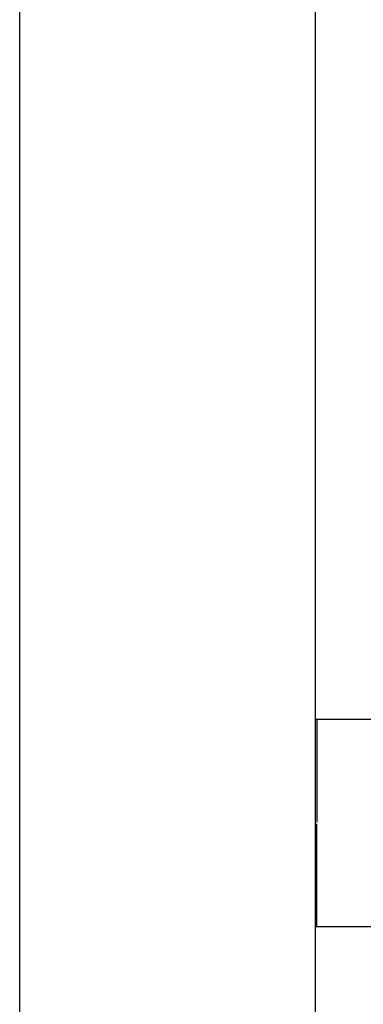
# Model space of a CAD drawing. Units: inches. Extents: x 311 to 815, y -527 to 136.
# Tile 15 of 21: x 311 to 388, y -210 to 13. Entities that reach past the tile are written whole.
import ezdxf

# ---------------------------------------------------------------- set-up
doc = ezdxf.new("R2010")
doc.units = ezdxf.units.IN
doc.header["$MEASUREMENT"] = 0
doc.layers.add('A-ANNO-DIMS', color=1, linetype='Continuous', lineweight=18)
doc.layers.add('A-ANNO-TTLB', color=1, linetype='Continuous', lineweight=25)
doc.styles.get("Standard").update_dxf_attribs({"font": 'arial.ttf'})
doc.dimstyles.get("Standard").update_dxf_attribs({"dimtxt": 0.18, "dimasz": 0.18, "dimexe": 0.18, "dimexo": 0.0625, "dimgap": 0.09, "dimtad": 0, "dimtih": 1, "dimtoh": 1, "dimdec": 1, "dimzin": 0, "dimdsep": 46, "dimlunit": 4, "dimtxsty": 'Standard', "dimcen": 0.09, "dimadec": 0, "dimazin": 0, "dimtfac": 1, "dimtdec": 1, "dimtofl": 0, "dimtmove": 0, "dimatfit": 3, "dimfxl": 1, "dimtolj": 1, "dimtzin": 0, "dimarcsym": 0})

# ---------------------------------------------------------------- blocks, each defined once
blk = doc.blocks.new('_ArchTick')
at = {"color": 0, "linetype": 'ByBlock', "const_width": 0.15}
blk.add_lwpolyline([(-0.5, -0.5), (0.5, 0.5)], dxfattribs=at)
blk = doc.blocks.new('_Oblique')
at = {"color": 0, "linetype": 'ByBlock', "lineweight": -2}
blk.add_line((-0.5, -0.5), (0.5, 0.5), dxfattribs=at)
blk = doc.blocks.new('*D3')
at = {"layer": 'A-ANNO-DIMS', "color": 0, "lineweight": -2, "transparency": 16777216}
for p, q in [((377.54, 21.87), (377.54, -221.61)), ((377.54, -482.13), (377.54, -238.65))]:
    blk.add_line(p, q, dxfattribs=at)
at = {"layer": 'Defpoints', "color": 0, "transparency": 16777216}
for p in [(410.32, 21.87), (377.54, -482.13), (410.32, -482.13)]:
    blk.add_point(p, dxfattribs=at)
at = {"layer": 'A-ANNO-DIMS', "color": 0, "lineweight": -2, "transparency": 16777216, "xscale": 9, "yscale": 9, "zscale": 9}
for name, p, rotation in [('_ArchTick', (377.54, 21.87), 90), ('_Oblique', (377.54, -482.13), 270)]:
    blk.add_blockref(name, p, dxfattribs=dict(at, rotation=rotation))
at = {"layer": 'A-ANNO-DIMS', "color": 0, "transparency": 16777216, "insert": (377.54, -230.13), "char_height": 9, "attachment_point": 5}
blk.add_mtext("\\A1;42'", dxfattribs=at)
blk = doc.blocks.new('*D32')
at = {"layer": 'A-ANNO-DIMS', "color": 0, "lineweight": -2, "transparency": 16777216}
for p, q in [((671.64, -145.62), (377.79, -145.62)), ((377.97, -145.8), (377.97, -168.9)), ((377.97, -192.37), (377.97, -169.27)), ((671.64, -192.55), (377.79, -192.55))]:
    blk.add_line(p, q, dxfattribs=at)
at = {"layer": 'A-ANNO-DIMS', "color": 0, "transparency": 16777216}
for points in [[(377.94, -145.8), (378, -145.8), (377.97, -145.62)], [(377.94, -192.37), (378, -192.37), (377.97, -192.55)]]:
    blk.add_solid(points, dxfattribs=at)
at = {"layer": 'Defpoints', "color": 0, "transparency": 16777216}
for p in [(671.7, -145.62), (377.97, -192.55), (671.7, -192.55)]:
    blk.add_point(p, dxfattribs=at)
at = {"layer": 'A-ANNO-DIMS', "color": 0, "transparency": 16777216, "insert": (377.97, -169.08), "char_height": 0.18, "attachment_point": 5}
blk.add_mtext('\\A1;3\'-11"', dxfattribs=at)

msp = doc.modelspace()

# ---------------------------------------------------------------- linework, layer by layer
at = {"layer": 'A-ANNO-TTLB'}
msp.add_lwpolyline([(310.67, 136.01), (815.43, 136.01), (815.43, -506.97), (310.67, -506.97)], close=True, dxfattribs=at)

# ---------------------------------------------------------------- dimensions: what is measured, and where the dimension line sits
at = {"layer": 'A-ANNO-DIMS'}
for base, p1, p2, override, picture, middle in [((377.54, -482.13), (410.32, 21.87), (410.32, -482.13), {"dimtxt": 9, "dimasz": 9, "dimgap": 4, "dimblk1": 'ArchTick', "dimblk2": 'Oblique', "dimsah": 1, "dimse1": 1, "dimse2": 1, "dimclrd": 0, "dimclre": 0, "dimclrt": 0}, '*D3', (377.54, -230.13)), ((377.97, -192.55), (671.7, -145.62), (671.7, -192.55), {"dimdec": 1, "dimlfac": 1, "dimrnd": 0, "dimzin": 1, "dimdsep": 46, "dimlunit": 4, "dimfrac": 2}, '*D32', (377.97, -169.08))]:
    dim = msp.add_linear_dim(base=base, p1=p1, p2=p2, angle=90, dimstyle='Standard', override=override, dxfattribs=at)
    dim.commit()
    dim.dimension.update_dxf_attribs({"geometry": picture, "text_midpoint": middle})

doc.saveas('drawing.dxf')
